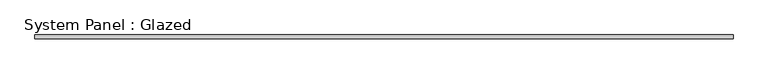
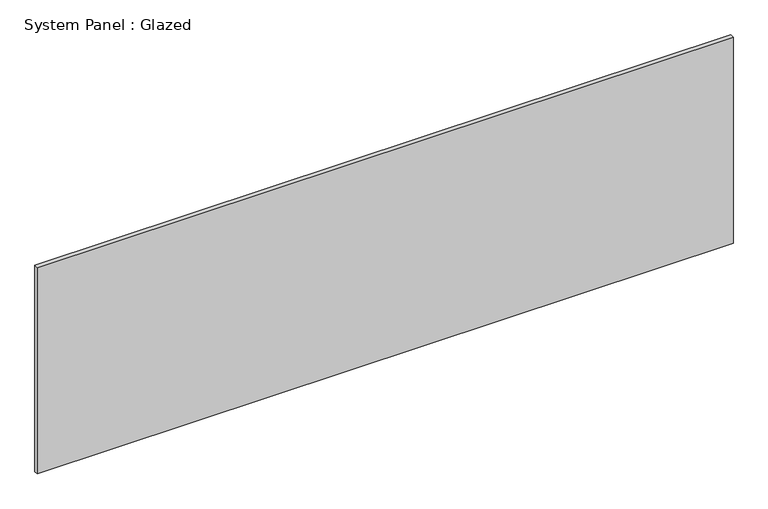
"""IFC4 building model written with IfcOpenShell, lengths in millimetres: plate geometry, System Panel : Glazed."""

from ifc_helpers import new_model, si_unit, origin, origin_with_axes, place, context, project, spatial, polyline, outline, extrude, source, transform, mapped, element, save


def system_panel_glazed_96c75d75(model_context):
    return source(origin(), model_context, "Body", "SweptSolid", [
        extrude(outline(polyline([(2330.45, 19.05), (-2330.45, 19.05), (-2330.45, 44.45), (2330.45, 44.45), (2330.45, 19.05)])), origin_with_axes(), (0.0, 0.0, 1.0), 1460.5),
    ])


if __name__ == "__main__":
    model = new_model("IFC4")
    model_context = context("Model", 3, world=origin())
    ifc_project = project(units=[si_unit("LENGTHUNIT", "METRE", prefix="MILLI")], contexts=[model_context])
    site = spatial("IfcSite", under=ifc_project)
    building = spatial("IfcBuilding", under=site)
    placement = place(None, origin())
    system_panel_glazed_shape = system_panel_glazed_96c75d75(model_context)
    element("IfcPlate", 1, ObjectType="System Panel : Glazed", at=placement, inside=building, context=model_context, shape_type="MappedRepresentation", body=[
        mapped(system_panel_glazed_shape, transform((0.0, 0.0, 0.0), x_axis=(1.0, 0.0, 0.0), y_axis=(0.0, 1.0, 0.0), z_axis=(0.0, 0.0, 1.0))),
    ])
    save(model, "model.ifc")

# Revit data of these elements
# Type "System Panel : Glazed"
#   Construction Type Id = "GSP4R"
#   Analytic Construction = "1/8 in Pilkington single glazing"
#   Visual Light Transmittance = 0.9
#   Solar Heat Gain Coefficient = 0.86
#   Heat Transfer Coefficient (U) = 1.18115 BTU/(h·ft²·°F)
# Element 1 (IfcPlate, "System Panel : Glazed")
#   Materials on its faces: "Glass"
# Materials
#   "Glass": class "Glass", colour RGB 0 128 192, transparency 0.75, Description = "Soda Lime Glass", Cost = 0
